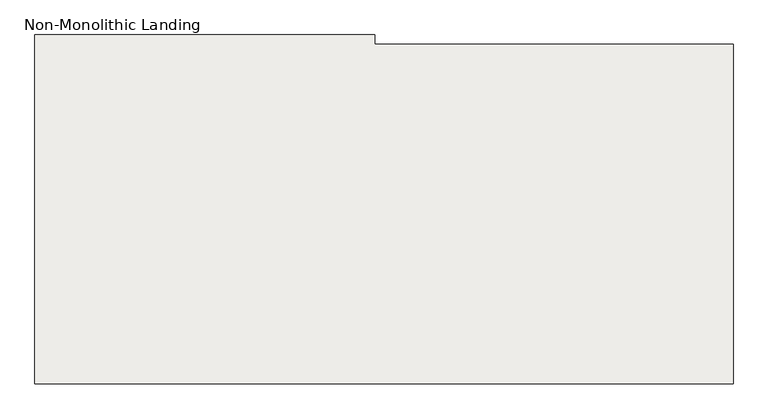
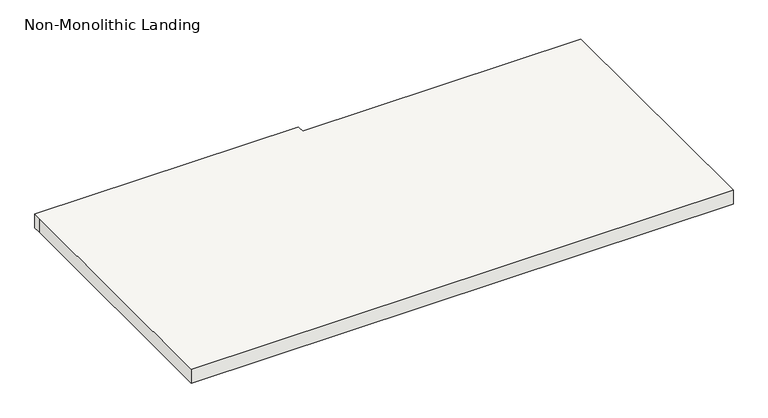
"""IFC4 building model written with IfcOpenShell, lengths in millimetres: slab geometry, Non-Monolithic Landing."""

from ifc_helpers import new_model, si_unit, origin, place, context, project, spatial, faceted_brep, source, transform, mapped, element, save


def non_monolithic_landing_b50a567b(model_context):
    return source(origin(), model_context, "Body", "Brep", [
        faceted_brep([(-3400.7137331, -6527.0593836, 7803.4118174), (-3400.7137331, -6552.4593836, 7778.0118174), (-4315.1137331, -6552.4593836, 7778.0118174), (-4315.1137331, -6527.0593836, 7803.4118174), (-4365.9137331, -6527.0593836, 7822.4618174), (-4365.9137331, -6501.6593836, 7822.4618174), (-5280.3137331, -6501.6593836, 7822.4618174), (-5280.3137331, -6527.0593836, 7822.4618174), (-5280.3137331, -7441.4593836, 7822.4618174), (-3400.7137331, -7441.4593836, 7822.4618174), (-3400.7137331, -6527.0593836, 7822.4618174), (-4315.1137331, -6552.4593836, 7771.6618174), (-3400.7137331, -6552.4593836, 7771.6618174), (-3400.7137331, -7441.4593836, 7771.6618174), (-5280.3137331, -7441.4593836, 7771.6618174), (-5280.3137331, -6527.0593836, 7771.6618174), (-5280.3137331, -6501.6593836, 7771.6618174), (-4365.9137331, -6501.6593836, 7771.6618174), (-4365.9137331, -6527.0593836, 7771.6618174), (-4315.1137331, -6527.0593836, 7771.6618174)], [[[0, 1, 2, 3]], [[4, 5, 6, 7, 8, 9, 10]], [[11, 12, 13, 14, 15, 16, 17, 18, 19]], [[12, 11, 2, 1]], [[11, 19, 3, 2]], [[4, 10, 0, 3, 19, 18]], [[5, 4, 18, 17]], [[6, 5, 17, 16]], [[7, 6, 16, 15]], [[8, 7, 15, 14]], [[9, 8, 14, 13]], [[10, 9, 13, 12, 1, 0]]]),
    ])


if __name__ == "__main__":
    model = new_model("IFC4")
    model_context = context("Model", 3, world=origin())
    ifc_project = project(units=[si_unit("LENGTHUNIT", "METRE", prefix="MILLI")], contexts=[model_context])
    site = spatial("IfcSite", under=ifc_project)
    building = spatial("IfcBuilding", under=site)
    placement = place(None, origin())
    non_monolithic_landing_shape = non_monolithic_landing_b50a567b(model_context)
    element("IfcSlab", 1, ObjectType="Non-Monolithic Landing", at=placement, inside=building, context=model_context, shape_type="MappedRepresentation", body=[
        mapped(non_monolithic_landing_shape, transform((0.0, 0.0, 0.0), x_axis=(1.0, 0.0, 0.0), y_axis=(0.0, 1.0, 0.0), z_axis=(0.0, 0.0, 1.0))),
    ])
    save(model, "model.ifc")
